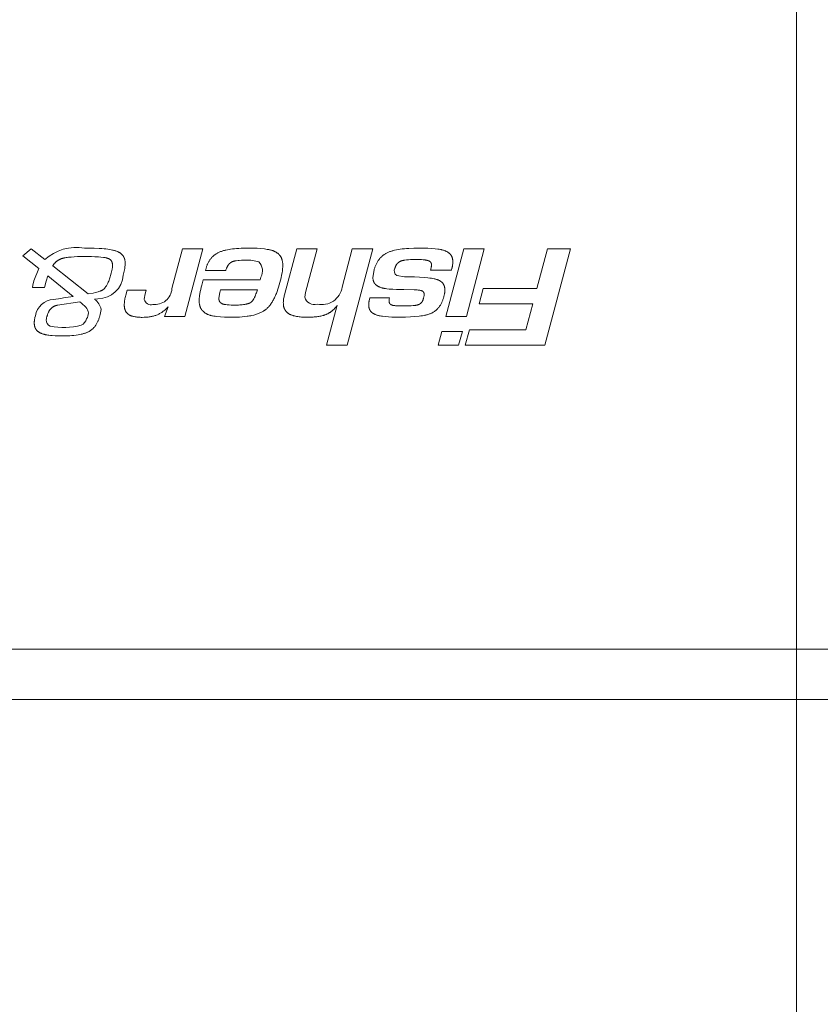
# Model space of a CAD drawing. Units: inches. Extents: x -1198 to -69, y -512 to 437.
# Tile 35 of 50: x -627.245 to -625.117, y 180.515 to 183.132. Entities that reach past the tile are written whole.
import ezdxf

# ---------------------------------------------------------------- set-up
doc = ezdxf.new("R2010")
doc.units = ezdxf.units.IN
doc.header["$MEASUREMENT"] = 0
for name, color, linetype, lineweight in [('0_Pen_No__7', 7, 'Continuous', 18), ('A-ANNO-DIMS', 2, 'Continuous', 18), ('A-EQPM', 60, 'Continuous', 18)]:
    doc.layers.add(name, color=color, linetype=linetype, lineweight=lineweight)
doc.styles.get("Standard").update_dxf_attribs({"font": 'arial.ttf'})
doc.dimstyles.get("Standard").update_dxf_attribs({"dimtxt": 6, "dimasz": 6, "dimexe": 0.18, "dimexo": 0.0625, "dimgap": 0.09, "dimtad": 0, "dimtih": 1, "dimtoh": 1, "dimdec": 0, "dimzin": 0, "dimdsep": 46, "dimlunit": 4, "dimtxsty": 'Standard', "dimblk": 'OBLIQUE', "dimcen": 0.09, "dimadec": 0, "dimazin": 0, "dimtfac": 1, "dimtdec": 0, "dimtofl": 0, "dimtmove": 0, "dimatfit": 3, "dimfxl": 1, "dimtolj": 1, "dimtzin": 0, "dimarcsym": 0})

# ---------------------------------------------------------------- blocks, each defined once
blk = doc.blocks.new('new block')
at = {"layer": '0_Pen_No__7'}
for p, q in [((-358.997, 99.109), (485.681, 99.109)), ((485.681, 95.73), (-358.997, 95.73)), ((-318.452, 68.7), (-316.721, 75.2)), ((-316.721, 75.2), (-311.349, 75.2)), ((-311.349, 75.2), (-311.629, 74.168)), ((-311.16, 74.266), (-310.904, 75.2)), ((-310.904, 75.2), (-309.527, 75.2)), ((-309.527, 75.2), (-309.782, 74.266)), ((-305.104, 68.7), (-303.373, 75.2)), ((-303.373, 75.2), (-301.997, 75.2)), ((-301.997, 75.2), (-302.715, 72.502)), ((-315.442, 74.168), (-315.906, 72.403)), ((-311.629, 74.168), (-315.442, 74.168)), ((-309.782, 74.266), (-311.16, 74.266)), ((-312.634, 68.7), (-311.429, 73.251)), ((-311.429, 73.251), (-310.05, 73.251)), ((-310.05, 73.251), (-311.257, 68.7)), ((-293.639, 68.7), (-292.433, 73.251)), ((-292.433, 73.251), (-291.056, 73.251)), ((-291.056, 73.251), (-291.311, 72.618)), ((-286.771, 72.786), (-286.716, 73.132)), ((-285.755, 72.627), (-285.462, 72.368)), ((-315.906, 72.403), (-312.288, 72.403)), ((-312.288, 72.403), (-312.567, 71.371)), ((-306.237, 72.004), (-306.225, 72.092)), ((-304.908, 72.004), (-306.237, 72.004)), ((-306.225, 72.092), (-306.213, 72.219)), ((-300.571, 71.634), (-300.522, 71.955)), ((-294.784, 71.634), (-294.723, 72.033)), ((-289.753, 71.731), (-289.691, 72.102)), ((-288.448, 71.819), (-288.533, 71.488)), ((-286.562, 72.059), (-286.329, 72.102)), ((-285.462, 72.368), (-285.335, 72.264)), ((-284.895, 71.907), (-283.174, 70.513)), ((-316.186, 71.371), (-316.892, 68.7)), ((-312.567, 71.371), (-316.186, 71.371)), ((-303.045, 71.283), (-303.727, 68.7)), ((-301.351, 68.7), (-300.571, 71.634)), ((-299.158, 71.789), (-299.974, 68.7)), ((-297.319, 71.458), (-294.833, 71.458)), ((-294.833, 71.458), (-294.784, 71.634)), ((-293.566, 71.146), (-293.663, 70.776)), ((-291.555, 71.379), (-292.26, 68.7)), ((-289.824, 71.488), (-289.753, 71.731)), ((-288.533, 71.488), (-289.824, 71.488)), ((-283.509, 69.837), (-285.894, 71.738)), ((-283.064, 70.877), (-282.962, 71.312)), ((-282.962, 71.312), (-282.141, 71.312)), ((-282.174, 71.152), (-282.242, 70.858)), ((-282.141, 71.312), (-282.174, 71.152)), ((-306.725, 70.503), (-307.261, 70.58)), ((-305.117, 70.62), (-305.202, 70.114)), ((-297.514, 70.776), (-297.561, 70.601)), ((-293.663, 70.776), (-297.514, 70.776)), ((-288.382, 70.016), (-288.272, 70.467)), ((-283.174, 70.513), (-283.064, 70.877)), ((-282.242, 70.858), (-282.564, 70.016)), ((-310.452, 70.006), (-310.417, 70.134)), ((-310.417, 70.134), (-309.003, 70.134)), ((-309.003, 70.134), (-309.04, 69.986)), ((-295.187, 70.152), (-293.822, 70.152)), ((-293.846, 70.065), (-293.858, 70.016)), ((-293.822, 70.152), (-293.846, 70.065)), ((-288.405, 69.686), (-288.382, 70.016)), ((-282.564, 70.016), (-281.486, 69.163)), ((-282.063, 68.7), (-282.973, 69.42)), ((-281.486, 69.163), (-282.063, 68.7)), ((-316.892, 68.7), (-318.452, 68.7)), ((-311.257, 68.7), (-312.634, 68.7)), ((-303.727, 68.7), (-305.104, 68.7)), ((-299.974, 68.7), (-301.351, 68.7)), ((-292.26, 68.7), (-293.639, 68.7))]:
    blk.add_line(p, q, dxfattribs=at)
blk.add_lwpolyline([(-333.701, 12.952), (460.296, 12.952), (460.296, 570.439), (-333.701, 570.439)], close=True, dxfattribs=at)
for points in [[(-286.716, 73.132), (-286.69, 73.224), (-286.662, 73.317), (-286.646, 73.362), (-286.63, 73.408), (-286.613, 73.453), (-286.595, 73.498), (-286.577, 73.543), (-286.557, 73.587), (-286.536, 73.63), (-286.514, 73.673), (-286.492, 73.716), (-286.468, 73.757), (-286.443, 73.799), (-286.417, 73.839), (-286.394, 73.873), (-286.37, 73.906), (-286.345, 73.938), (-286.32, 73.97), (-286.294, 74.001), (-286.266, 74.031), (-286.238, 74.06), (-286.209, 74.089), (-286.181, 74.115), (-286.152, 74.14), (-286.122, 74.164), (-286.091, 74.187), (-286.06, 74.209), (-286.028, 74.23), (-285.996, 74.25), (-285.963, 74.269), (-285.924, 74.29), (-285.885, 74.309), (-285.846, 74.327), (-285.806, 74.344), (-285.765, 74.36), (-285.724, 74.375), (-285.683, 74.389), (-285.641, 74.402), (-285.59, 74.417), (-285.538, 74.431), (-285.486, 74.444), (-285.434, 74.456), (-285.329, 74.478), (-285.223, 74.496), (-285.084, 74.517), (-284.943, 74.534), (-284.803, 74.547), (-284.662, 74.557), (-284.521, 74.564), (-284.379, 74.568), (-284.097, 74.572)], [(-284.097, 74.572), (-283.885, 74.569), (-283.673, 74.56), (-283.461, 74.545), (-283.355, 74.535), (-283.249, 74.523), (-283.177, 74.513), (-283.105, 74.502), (-283.033, 74.489), (-282.997, 74.481), (-282.962, 74.473), (-282.926, 74.464), (-282.891, 74.455), (-282.856, 74.444), (-282.821, 74.433), (-282.787, 74.42), (-282.753, 74.407), (-282.719, 74.393), (-282.686, 74.377), (-282.662, 74.365), (-282.639, 74.353), (-282.616, 74.34), (-282.594, 74.326), (-282.572, 74.312), (-282.55, 74.297), (-282.529, 74.282), (-282.508, 74.266), (-282.488, 74.249), (-282.478, 74.24), (-282.469, 74.232), (-282.459, 74.223), (-282.45, 74.214), (-282.441, 74.204), (-282.432, 74.195), (-282.423, 74.186), (-282.415, 74.176), (-282.407, 74.166), (-282.399, 74.156), (-282.391, 74.146), (-282.383, 74.135), (-282.376, 74.125), (-282.369, 74.114), (-282.362, 74.103), (-282.355, 74.091), (-282.349, 74.08), (-282.343, 74.068), (-282.337, 74.056), (-282.331, 74.044), (-282.326, 74.032), (-282.32, 74.02), (-282.315, 74.007), (-282.311, 73.995), (-282.306, 73.982), (-282.302, 73.969), (-282.298, 73.956), (-282.294, 73.943), (-282.291, 73.93), (-282.288, 73.917), (-282.282, 73.891), (-282.277, 73.864), (-282.273, 73.837), (-282.269, 73.81), (-282.267, 73.782), (-282.265, 73.755), (-282.264, 73.728), (-282.263, 73.701), (-282.263, 73.669), (-282.265, 73.638), (-282.267, 73.606), (-282.269, 73.575), (-282.273, 73.544), (-282.277, 73.513), (-282.282, 73.482), (-282.287, 73.451), (-282.299, 73.39), (-282.312, 73.329), (-282.342, 73.207)], [(-309.904, 71.926), (-309.878, 72.017), (-309.864, 72.062), (-309.849, 72.107), (-309.833, 72.152), (-309.816, 72.196), (-309.798, 72.24), (-309.78, 72.283), (-309.76, 72.326), (-309.739, 72.369), (-309.717, 72.411), (-309.694, 72.452), (-309.67, 72.493), (-309.645, 72.533), (-309.618, 72.572), (-309.591, 72.61), (-309.566, 72.643), (-309.54, 72.676), (-309.512, 72.707), (-309.484, 72.738), (-309.455, 72.768), (-309.426, 72.797), (-309.395, 72.825), (-309.363, 72.852), (-309.331, 72.878), (-309.298, 72.902), (-309.265, 72.926), (-309.23, 72.948), (-309.196, 72.969), (-309.16, 72.99), (-309.124, 73.009), (-309.087, 73.027), (-309.039, 73.05), (-308.989, 73.071), (-308.939, 73.091), (-308.888, 73.108), (-308.837, 73.125), (-308.785, 73.14), (-308.732, 73.154), (-308.68, 73.167), (-308.627, 73.179), (-308.573, 73.19), (-308.466, 73.209), (-308.359, 73.225), (-308.251, 73.239), (-307.955, 73.271), (-307.661, 73.292), (-307.323, 73.305), (-306.956, 73.31), (-306.678, 73.308), (-306.4, 73.299), (-306.169, 73.285), (-305.939, 73.266), (-305.777, 73.248), (-305.696, 73.237), (-305.615, 73.224), (-305.575, 73.216), (-305.535, 73.207), (-305.496, 73.198), (-305.456, 73.188), (-305.416, 73.176), (-305.377, 73.164), (-305.338, 73.15), (-305.299, 73.135), (-305.274, 73.124), (-305.249, 73.113), (-305.224, 73.102), (-305.199, 73.09), (-305.175, 73.077), (-305.151, 73.063), (-305.128, 73.049), (-305.105, 73.034), (-305.094, 73.026), (-305.083, 73.019), (-305.072, 73.01), (-305.062, 73.002), (-305.051, 72.994), (-305.041, 72.985), (-305.031, 72.976), (-305.021, 72.967), (-305.011, 72.958), (-305.002, 72.949), (-304.993, 72.939), (-304.984, 72.929), (-304.975, 72.919), (-304.967, 72.909), (-304.959, 72.899), (-304.951, 72.888), (-304.944, 72.877), (-304.937, 72.866), (-304.93, 72.855), (-304.923, 72.844), (-304.917, 72.832), (-304.911, 72.821), (-304.905, 72.809), (-304.899, 72.797), (-304.894, 72.785), (-304.889, 72.772), (-304.884, 72.76), (-304.88, 72.747), (-304.875, 72.735), (-304.871, 72.722), (-304.868, 72.709), (-304.864, 72.696), (-304.861, 72.683), (-304.858, 72.67), (-304.852, 72.643), (-304.847, 72.616), (-304.843, 72.589), (-304.84, 72.562), (-304.838, 72.535), (-304.837, 72.508), (-304.836, 72.481), (-304.836, 72.45), (-304.836, 72.42), (-304.838, 72.389), (-304.84, 72.359), (-304.843, 72.329), (-304.847, 72.299), (-304.852, 72.269), (-304.856, 72.239), (-304.867, 72.18), (-304.88, 72.121), (-304.908, 72.004)], [(-302.715, 72.502), (-302.674, 72.555), (-302.631, 72.607), (-302.588, 72.659), (-302.542, 72.709), (-302.495, 72.757), (-302.447, 72.804), (-302.422, 72.827), (-302.396, 72.85), (-302.371, 72.872), (-302.345, 72.893), (-302.321, 72.912), (-302.298, 72.93), (-302.274, 72.947), (-302.249, 72.965), (-302.225, 72.981), (-302.2, 72.998), (-302.175, 73.014), (-302.149, 73.029), (-302.124, 73.044), (-302.098, 73.059), (-302.072, 73.073), (-302.045, 73.086), (-302.018, 73.099), (-301.991, 73.112), (-301.964, 73.124), (-301.937, 73.135), (-301.905, 73.147), (-301.873, 73.159), (-301.841, 73.17), (-301.809, 73.181), (-301.776, 73.191), (-301.743, 73.2), (-301.677, 73.217), (-301.611, 73.231), (-301.544, 73.244), (-301.476, 73.256), (-301.409, 73.266), (-301.327, 73.277), (-301.244, 73.286), (-301.162, 73.293), (-301.079, 73.299), (-300.893, 73.307), (-300.706, 73.31), (-300.505, 73.307), (-300.404, 73.302), (-300.304, 73.296), (-300.218, 73.288), (-300.133, 73.279), (-300.048, 73.267), (-299.963, 73.254), (-299.897, 73.241), (-299.833, 73.227), (-299.8, 73.22), (-299.768, 73.211), (-299.736, 73.202), (-299.705, 73.193), (-299.673, 73.182), (-299.642, 73.171), (-299.611, 73.159), (-299.581, 73.146), (-299.551, 73.133), (-299.521, 73.118), (-299.492, 73.102), (-299.477, 73.094), (-299.463, 73.085), (-299.441, 73.071), (-299.419, 73.057), (-299.397, 73.041), (-299.376, 73.025), (-299.356, 73.009), (-299.335, 72.992), (-299.316, 72.974), (-299.297, 72.955), (-299.278, 72.936), (-299.261, 72.917), (-299.244, 72.897), (-299.236, 72.887), (-299.228, 72.876), (-299.22, 72.866), (-299.212, 72.855), (-299.205, 72.844), (-299.197, 72.833), (-299.19, 72.822), (-299.184, 72.811), (-299.177, 72.8), (-299.171, 72.788), (-299.164, 72.776), (-299.158, 72.763), (-299.152, 72.751), (-299.146, 72.738), (-299.14, 72.725), (-299.135, 72.712), (-299.13, 72.698), (-299.125, 72.685), (-299.121, 72.672), (-299.116, 72.658), (-299.109, 72.631), (-299.101, 72.603), (-299.095, 72.575), (-299.09, 72.547), (-299.085, 72.518), (-299.082, 72.49), (-299.079, 72.461), (-299.076, 72.433), (-299.075, 72.404), (-299.074, 72.375), (-299.073, 72.346), (-299.073, 72.311), (-299.074, 72.275), (-299.076, 72.239), (-299.079, 72.204), (-299.082, 72.169), (-299.086, 72.134), (-299.091, 72.099), (-299.096, 72.064), (-299.109, 71.994), (-299.123, 71.925), (-299.14, 71.857), (-299.158, 71.789)], [(-298.842, 70.97), (-298.801, 71.12), (-298.757, 71.27), (-298.71, 71.418), (-298.659, 71.565), (-298.603, 71.711), (-298.574, 71.783), (-298.543, 71.854), (-298.511, 71.925), (-298.477, 71.995), (-298.442, 72.064), (-298.406, 72.133), (-298.376, 72.186), (-298.345, 72.239), (-298.313, 72.292), (-298.28, 72.343), (-298.246, 72.394), (-298.211, 72.444), (-298.174, 72.493), (-298.135, 72.54), (-298.101, 72.581), (-298.066, 72.62), (-298.029, 72.659), (-297.992, 72.696), (-297.953, 72.733), (-297.913, 72.767), (-297.893, 72.784), (-297.872, 72.801), (-297.851, 72.817), (-297.83, 72.833), (-297.808, 72.849), (-297.785, 72.864), (-297.763, 72.879), (-297.739, 72.894), (-297.692, 72.922), (-297.645, 72.948), (-297.596, 72.974), (-297.546, 72.997), (-297.496, 73.02), (-297.446, 73.041), (-297.385, 73.064), (-297.324, 73.086), (-297.263, 73.107), (-297.201, 73.126), (-297.139, 73.144), (-297.076, 73.16), (-296.95, 73.19), (-296.869, 73.207), (-296.787, 73.222), (-296.705, 73.236), (-296.622, 73.249), (-296.457, 73.27), (-296.291, 73.286), (-296.125, 73.297), (-295.958, 73.305), (-295.625, 73.31)], [(-295.625, 73.31), (-295.36, 73.306), (-295.094, 73.296), (-294.828, 73.278), (-294.562, 73.251), (-294.474, 73.241), (-294.386, 73.229), (-294.299, 73.214), (-294.255, 73.205), (-294.212, 73.196), (-294.169, 73.186), (-294.127, 73.174), (-294.085, 73.161), (-294.043, 73.147), (-294.002, 73.132), (-293.982, 73.124), (-293.962, 73.115), (-293.942, 73.106), (-293.922, 73.097), (-293.902, 73.087), (-293.882, 73.077), (-293.855, 73.062), (-293.827, 73.045), (-293.8, 73.028), (-293.774, 73.01), (-293.748, 72.991), (-293.723, 72.972), (-293.699, 72.951), (-293.675, 72.93), (-293.652, 72.908), (-293.641, 72.897), (-293.63, 72.886), (-293.619, 72.874), (-293.608, 72.862), (-293.598, 72.85), (-293.588, 72.838), (-293.578, 72.826), (-293.568, 72.813), (-293.559, 72.801), (-293.55, 72.788), (-293.541, 72.775), (-293.533, 72.762), (-293.525, 72.748), (-293.517, 72.735), (-293.508, 72.719), (-293.5, 72.704), (-293.492, 72.688), (-293.484, 72.672), (-293.477, 72.655), (-293.47, 72.639), (-293.464, 72.622), (-293.458, 72.606), (-293.452, 72.589), (-293.447, 72.572), (-293.442, 72.555), (-293.437, 72.537), (-293.432, 72.52), (-293.428, 72.503), (-293.42, 72.467), (-293.414, 72.432), (-293.409, 72.396), (-293.404, 72.36), (-293.401, 72.324), (-293.398, 72.288), (-293.396, 72.251), (-293.395, 72.215), (-293.395, 72.179), (-293.396, 72.122), (-293.398, 72.065), (-293.402, 72.009), (-293.407, 71.953), (-293.413, 71.897), (-293.42, 71.842), (-293.437, 71.731), (-293.464, 71.584), (-293.495, 71.437), (-293.529, 71.291), (-293.566, 71.146)], [(-291.311, 72.618), (-291.264, 72.662), (-291.217, 72.706), (-291.168, 72.749), (-291.119, 72.792), (-291.069, 72.833), (-291.018, 72.873), (-290.966, 72.911), (-290.913, 72.949), (-290.866, 72.98), (-290.819, 73.011), (-290.771, 73.04), (-290.722, 73.068), (-290.673, 73.094), (-290.623, 73.119), (-290.572, 73.142), (-290.521, 73.164), (-290.468, 73.184), (-290.414, 73.203), (-290.359, 73.219), (-290.304, 73.235), (-290.249, 73.248), (-290.193, 73.26), (-290.137, 73.271), (-290.081, 73.281), (-290.017, 73.29), (-289.953, 73.298), (-289.889, 73.304), (-289.825, 73.31), (-289.755, 73.314), (-289.685, 73.317), (-289.545, 73.319), (-289.472, 73.319), (-289.4, 73.317), (-289.327, 73.313), (-289.255, 73.307), (-289.192, 73.301), (-289.13, 73.293), (-289.068, 73.283), (-289.006, 73.271), (-288.956, 73.26), (-288.907, 73.247), (-288.883, 73.24), (-288.859, 73.233), (-288.835, 73.225), (-288.811, 73.216), (-288.787, 73.207), (-288.764, 73.197), (-288.741, 73.187), (-288.718, 73.176), (-288.696, 73.164), (-288.674, 73.151), (-288.663, 73.145), (-288.653, 73.138), (-288.642, 73.131), (-288.632, 73.124), (-288.615, 73.111), (-288.598, 73.098), (-288.581, 73.085), (-288.565, 73.07), (-288.549, 73.056), (-288.534, 73.041), (-288.52, 73.025), (-288.505, 73.009), (-288.492, 72.992), (-288.478, 72.975), (-288.466, 72.958), (-288.454, 72.94), (-288.442, 72.922), (-288.432, 72.904), (-288.422, 72.885), (-288.412, 72.866), (-288.407, 72.855), (-288.402, 72.844), (-288.397, 72.832), (-288.393, 72.821), (-288.389, 72.81), (-288.385, 72.798), (-288.381, 72.786), (-288.377, 72.775), (-288.37, 72.751), (-288.364, 72.727), (-288.359, 72.703), (-288.355, 72.679), (-288.351, 72.654), (-288.347, 72.63), (-288.345, 72.605), (-288.343, 72.58), (-288.341, 72.556), (-288.34, 72.531), (-288.339, 72.481), (-288.34, 72.439), (-288.341, 72.396), (-288.344, 72.354), (-288.347, 72.312), (-288.352, 72.27), (-288.357, 72.229), (-288.363, 72.187), (-288.37, 72.145), (-288.386, 72.063), (-288.405, 71.981), (-288.426, 71.9), (-288.448, 71.819)], [(-285.335, 72.264), (-283.828, 72.5), (-283.806, 72.504), (-283.784, 72.508), (-283.762, 72.514), (-283.739, 72.519), (-283.717, 72.526), (-283.695, 72.533), (-283.673, 72.541), (-283.652, 72.549), (-283.631, 72.558), (-283.609, 72.567), (-283.59, 72.577), (-283.572, 72.587), (-283.553, 72.597), (-283.535, 72.608), (-283.517, 72.62), (-283.5, 72.632), (-283.483, 72.644), (-283.466, 72.657), (-283.45, 72.67), (-283.435, 72.684), (-283.42, 72.697), (-283.405, 72.712), (-283.391, 72.726), (-283.377, 72.741), (-283.364, 72.756), (-283.351, 72.772), (-283.338, 72.787), (-283.326, 72.804), (-283.313, 72.82), (-283.302, 72.837), (-283.29, 72.853), (-283.279, 72.871), (-283.268, 72.888), (-283.258, 72.905), (-283.248, 72.923), (-283.239, 72.94), (-283.22, 72.976), (-283.204, 73.012), (-283.188, 73.049), (-283.173, 73.086), (-283.159, 73.123), (-283.146, 73.161), (-283.134, 73.199), (-283.124, 73.235), (-283.115, 73.27), (-283.097, 73.342), (-283.082, 73.414), (-283.068, 73.487)], [(-307.236, 72.55), (-307.388, 72.549), (-307.54, 72.544), (-307.693, 72.536), (-307.846, 72.525), (-307.939, 72.516), (-307.986, 72.511), (-308.009, 72.507), (-308.032, 72.503), (-308.055, 72.499), (-308.078, 72.494), (-308.101, 72.489), (-308.123, 72.483), (-308.145, 72.476), (-308.167, 72.469), (-308.189, 72.461), (-308.2, 72.457), (-308.211, 72.452), (-308.224, 72.446), (-308.238, 72.44), (-308.251, 72.433), (-308.264, 72.426), (-308.277, 72.418), (-308.29, 72.411), (-308.302, 72.403), (-308.315, 72.394), (-308.327, 72.386), (-308.338, 72.377), (-308.35, 72.367), (-308.361, 72.358), (-308.372, 72.348), (-308.383, 72.337), (-308.393, 72.326), (-308.403, 72.315), (-308.413, 72.304), (-308.422, 72.292), (-308.431, 72.28), (-308.439, 72.267), (-308.447, 72.255), (-308.455, 72.242), (-308.463, 72.228), (-308.47, 72.215), (-308.477, 72.201), (-308.483, 72.188), (-308.489, 72.174), (-308.495, 72.159), (-308.5, 72.145), (-308.505, 72.131), (-308.51, 72.117), (-308.515, 72.102), (-308.522, 72.075), (-308.529, 72.048), (-308.535, 72.02), (-308.568, 71.844), (-308.572, 71.825), (-308.575, 71.807), (-308.577, 71.788), (-308.578, 71.769), (-308.578, 71.75), (-308.577, 71.736), (-308.576, 71.721), (-308.574, 71.711), (-308.572, 71.701), (-308.57, 71.691), (-308.567, 71.681), (-308.564, 71.671), (-308.561, 71.662), (-308.557, 71.652), (-308.552, 71.643), (-308.548, 71.634), (-308.543, 71.625), (-308.538, 71.616), (-308.532, 71.608), (-308.526, 71.6), (-308.516, 71.589), (-308.508, 71.58), (-308.499, 71.572), (-308.489, 71.563), (-308.478, 71.556), (-308.467, 71.549), (-308.455, 71.542), (-308.444, 71.536), (-308.431, 71.531), (-308.413, 71.523), (-308.4, 71.519), (-308.387, 71.514), (-308.374, 71.511), (-308.36, 71.507), (-308.347, 71.504), (-308.32, 71.498), (-308.294, 71.493), (-308.268, 71.488), (-308.243, 71.484), (-308.217, 71.48), (-308.166, 71.474), (-308.115, 71.47), (-308.064, 71.466), (-307.913, 71.461), (-307.2, 71.448)], [(-306.213, 72.219), (-306.213, 72.23), (-306.213, 72.242), (-306.214, 72.253), (-306.215, 72.265), (-306.217, 72.277), (-306.219, 72.288), (-306.221, 72.3), (-306.224, 72.311), (-306.227, 72.322), (-306.23, 72.333), (-306.234, 72.344), (-306.239, 72.354), (-306.244, 72.365), (-306.249, 72.375), (-306.255, 72.384), (-306.261, 72.394), (-306.268, 72.402), (-306.275, 72.411), (-306.283, 72.419), (-306.291, 72.426), (-306.299, 72.433), (-306.308, 72.44), (-306.317, 72.447), (-306.326, 72.453), (-306.336, 72.459), (-306.346, 72.465), (-306.356, 72.47), (-306.366, 72.475), (-306.376, 72.48), (-306.387, 72.484), (-306.397, 72.488), (-306.408, 72.492), (-306.427, 72.498), (-306.445, 72.504), (-306.464, 72.509), (-306.483, 72.513), (-306.502, 72.517), (-306.521, 72.52), (-306.54, 72.523), (-306.559, 72.526), (-306.597, 72.529), (-306.635, 72.532), (-306.974, 72.546), (-307.236, 72.55)], [(-295.807, 72.492), (-295.973, 72.49), (-296.056, 72.488), (-296.139, 72.484), (-296.222, 72.478), (-296.304, 72.47), (-296.386, 72.46), (-296.468, 72.448), (-296.526, 72.437), (-296.585, 72.424), (-296.614, 72.417), (-296.643, 72.41), (-296.671, 72.401), (-296.7, 72.392), (-296.722, 72.385), (-296.744, 72.377), (-296.765, 72.369), (-296.787, 72.36), (-296.797, 72.355), (-296.808, 72.35), (-296.818, 72.345), (-296.828, 72.339), (-296.838, 72.334), (-296.848, 72.328), (-296.858, 72.322), (-296.867, 72.315), (-296.876, 72.309), (-296.885, 72.303), (-296.893, 72.296), (-296.902, 72.29), (-296.91, 72.283), (-296.918, 72.275), (-296.926, 72.268), (-296.934, 72.261), (-296.941, 72.253), (-296.949, 72.245), (-296.964, 72.229), (-296.978, 72.213), (-296.992, 72.196), (-297.008, 72.175), (-297.024, 72.153), (-297.04, 72.13), (-297.054, 72.107), (-297.069, 72.084), (-297.082, 72.061), (-297.109, 72.013), (-297.126, 71.98), (-297.142, 71.947), (-297.158, 71.913), (-297.173, 71.879), (-297.201, 71.811), (-297.228, 71.741), (-297.253, 71.671), (-297.276, 71.6), (-297.319, 71.458)], [(-294.723, 72.033), (-294.723, 72.048), (-294.724, 72.063), (-294.725, 72.079), (-294.726, 72.094), (-294.728, 72.11), (-294.73, 72.125), (-294.732, 72.14), (-294.736, 72.155), (-294.739, 72.17), (-294.743, 72.185), (-294.748, 72.2), (-294.753, 72.214), (-294.759, 72.228), (-294.766, 72.242), (-294.773, 72.255), (-294.781, 72.268), (-294.789, 72.279), (-294.797, 72.29), (-294.806, 72.3), (-294.815, 72.31), (-294.825, 72.32), (-294.835, 72.329), (-294.846, 72.338), (-294.857, 72.347), (-294.868, 72.355), (-294.88, 72.363), (-294.891, 72.37), (-294.904, 72.377), (-294.916, 72.384), (-294.928, 72.391), (-294.941, 72.397), (-294.954, 72.403), (-294.963, 72.407), (-294.973, 72.411), (-294.992, 72.418), (-295.012, 72.425), (-295.032, 72.431), (-295.052, 72.436), (-295.072, 72.441), (-295.092, 72.445), (-295.113, 72.449), (-295.133, 72.453), (-295.154, 72.456), (-295.195, 72.461), (-295.277, 72.469), (-295.41, 72.479), (-295.542, 72.486), (-295.675, 72.491), (-295.807, 72.492)], [(-307.261, 70.58), (-307.93, 70.588), (-308.264, 70.602), (-308.598, 70.625), (-308.835, 70.648), (-308.954, 70.663), (-309.072, 70.68), (-309.159, 70.695), (-309.246, 70.712), (-309.29, 70.722), (-309.333, 70.732), (-309.375, 70.744), (-309.418, 70.757), (-309.45, 70.767), (-309.481, 70.779), (-309.513, 70.791), (-309.543, 70.804), (-309.574, 70.818), (-309.604, 70.833), (-309.619, 70.841), (-309.634, 70.849), (-309.648, 70.857), (-309.663, 70.866), (-309.675, 70.874), (-309.687, 70.882), (-309.699, 70.89), (-309.711, 70.898), (-309.723, 70.907), (-309.734, 70.916), (-309.746, 70.925), (-309.757, 70.934), (-309.768, 70.944), (-309.778, 70.954), (-309.789, 70.964), (-309.799, 70.974), (-309.809, 70.984), (-309.819, 70.995), (-309.828, 71.006), (-309.837, 71.017), (-309.846, 71.029), (-309.854, 71.04), (-309.862, 71.052), (-309.87, 71.064), (-309.877, 71.076), (-309.884, 71.088), (-309.891, 71.101), (-309.898, 71.113), (-309.904, 71.126), (-309.91, 71.139), (-309.916, 71.152), (-309.921, 71.165), (-309.926, 71.179), (-309.931, 71.192), (-309.936, 71.206), (-309.94, 71.22), (-309.944, 71.234), (-309.948, 71.248), (-309.952, 71.262), (-309.955, 71.276), (-309.961, 71.304), (-309.966, 71.333), (-309.97, 71.362), (-309.973, 71.39), (-309.976, 71.419), (-309.977, 71.448), (-309.977, 71.479), (-309.977, 71.509), (-309.976, 71.54), (-309.973, 71.57), (-309.97, 71.6), (-309.967, 71.63), (-309.963, 71.66), (-309.958, 71.69), (-309.946, 71.75), (-309.933, 71.809), (-309.904, 71.926)], [(-307.2, 71.448), (-306.952, 71.446), (-306.705, 71.438), (-306.457, 71.425), (-306.209, 71.405), (-306.049, 71.387), (-305.969, 71.376), (-305.89, 71.363), (-305.851, 71.355), (-305.811, 71.347), (-305.772, 71.337), (-305.733, 71.327), (-305.694, 71.315), (-305.656, 71.303), (-305.617, 71.289), (-305.579, 71.274), (-305.554, 71.263), (-305.529, 71.252), (-305.504, 71.24), (-305.48, 71.228), (-305.455, 71.215), (-305.432, 71.201), (-305.409, 71.187), (-305.386, 71.171), (-305.375, 71.164), (-305.364, 71.156), (-305.353, 71.147), (-305.342, 71.139), (-305.332, 71.13), (-305.322, 71.122), (-305.312, 71.113), (-305.302, 71.103), (-305.292, 71.094), (-305.283, 71.084), (-305.274, 71.075), (-305.265, 71.065), (-305.256, 71.055), (-305.248, 71.044), (-305.24, 71.034), (-305.232, 71.023), (-305.225, 71.012), (-305.217, 71.001), (-305.211, 70.99), (-305.204, 70.978), (-305.198, 70.967), (-305.191, 70.955), (-305.186, 70.943), (-305.18, 70.931), (-305.175, 70.919), (-305.17, 70.907), (-305.165, 70.895), (-305.16, 70.882), (-305.156, 70.87), (-305.152, 70.857), (-305.148, 70.844), (-305.144, 70.831), (-305.141, 70.818), (-305.138, 70.805), (-305.135, 70.792), (-305.132, 70.779), (-305.127, 70.752), (-305.123, 70.726), (-305.12, 70.699), (-305.118, 70.673), (-305.117, 70.647), (-305.117, 70.62)], [(-285.894, 71.738), (-286.234, 71.675), (-286.403, 71.638), (-286.486, 71.617), (-286.57, 71.594), (-286.625, 71.577), (-286.679, 71.559), (-286.706, 71.549), (-286.733, 71.539), (-286.76, 71.528), (-286.786, 71.517), (-286.806, 71.507), (-286.826, 71.497), (-286.846, 71.487), (-286.865, 71.476), (-286.884, 71.465), (-286.893, 71.459), (-286.902, 71.453), (-286.911, 71.447), (-286.92, 71.44), (-286.929, 71.434), (-286.937, 71.427), (-286.946, 71.42), (-286.955, 71.412), (-286.963, 71.405), (-286.971, 71.397), (-286.979, 71.389), (-286.987, 71.381), (-287.003, 71.364), (-287.018, 71.347), (-287.032, 71.329), (-287.046, 71.311), (-287.06, 71.293), (-287.078, 71.268), (-287.095, 71.243), (-287.112, 71.218), (-287.128, 71.193), (-287.159, 71.142), (-287.188, 71.09), (-287.207, 71.055), (-287.225, 71.02), (-287.258, 70.949), (-287.29, 70.876), (-287.32, 70.803), (-287.347, 70.729), (-287.372, 70.654), (-287.396, 70.579), (-287.417, 70.503)], [(-293.858, 70.016), (-293.869, 69.973), (-293.882, 69.929), (-293.895, 69.886), (-293.91, 69.844), (-293.925, 69.801), (-293.942, 69.759), (-293.96, 69.717), (-293.978, 69.676), (-293.998, 69.635), (-294.018, 69.595), (-294.04, 69.555), (-294.063, 69.516), (-294.087, 69.478), (-294.112, 69.441), (-294.139, 69.404), (-294.166, 69.368), (-294.193, 69.335), (-294.221, 69.303), (-294.25, 69.271), (-294.28, 69.241), (-294.311, 69.211), (-294.343, 69.182), (-294.375, 69.154), (-294.409, 69.127), (-294.443, 69.101), (-294.478, 69.076), (-294.513, 69.052), (-294.549, 69.028), (-294.586, 69.006), (-294.623, 68.985), (-294.66, 68.964), (-294.698, 68.945), (-294.746, 68.922), (-294.795, 68.9), (-294.844, 68.88), (-294.894, 68.862), (-294.944, 68.844), (-294.994, 68.828), (-295.045, 68.813), (-295.097, 68.799), (-295.148, 68.786), (-295.2, 68.774), (-295.305, 68.753), (-295.41, 68.734), (-295.515, 68.718), (-295.651, 68.699), (-295.788, 68.684), (-295.924, 68.671), (-296.06, 68.661), (-296.22, 68.653), (-296.379, 68.647), (-296.698, 68.642), (-297, 68.645), (-297.151, 68.65), (-297.301, 68.658), (-297.553, 68.677), (-297.806, 68.703), (-297.899, 68.714), (-297.992, 68.728), (-298.084, 68.743), (-298.13, 68.752), (-298.175, 68.762), (-298.221, 68.773), (-298.265, 68.785), (-298.31, 68.798), (-298.354, 68.813), (-298.398, 68.829), (-298.419, 68.837), (-298.441, 68.846), (-298.462, 68.856), (-298.483, 68.866), (-298.504, 68.876), (-298.525, 68.887), (-298.554, 68.902), (-298.583, 68.919), (-298.611, 68.937), (-298.639, 68.955), (-298.666, 68.975), (-298.692, 68.995), (-298.718, 69.016), (-298.743, 69.038), (-298.755, 69.049), (-298.767, 69.061), (-298.779, 69.072), (-298.791, 69.084), (-298.802, 69.096), (-298.813, 69.109), (-298.824, 69.121), (-298.834, 69.134), (-298.845, 69.147), (-298.855, 69.16), (-298.864, 69.173), (-298.874, 69.186), (-298.883, 69.2), (-298.892, 69.214), (-298.901, 69.228), (-298.909, 69.242), (-298.917, 69.257), (-298.925, 69.272), (-298.933, 69.288), (-298.94, 69.304), (-298.947, 69.32), (-298.954, 69.336), (-298.96, 69.352), (-298.966, 69.369), (-298.972, 69.385), (-298.978, 69.402), (-298.988, 69.435), (-298.997, 69.469), (-299.004, 69.503), (-299.012, 69.542), (-299.019, 69.582), (-299.024, 69.621), (-299.029, 69.661), (-299.032, 69.701), (-299.035, 69.741), (-299.036, 69.781), (-299.036, 69.82), (-299.035, 69.882), (-299.033, 69.943), (-299.028, 70.004), (-299.022, 70.065), (-299.015, 70.126), (-299.007, 70.187), (-298.988, 70.309), (-298.957, 70.475), (-298.922, 70.641), (-298.842, 70.97)], [(-287.417, 70.503), (-287.464, 70.331), (-287.506, 70.158), (-287.524, 70.07), (-287.532, 70.026), (-287.539, 69.982), (-287.544, 69.938), (-287.546, 69.915), (-287.548, 69.893), (-287.549, 69.871), (-287.55, 69.848), (-287.55, 69.825), (-287.549, 69.802), (-287.549, 69.782), (-287.547, 69.761), (-287.545, 69.74), (-287.542, 69.719), (-287.539, 69.698), (-287.535, 69.677), (-287.531, 69.657), (-287.528, 69.647), (-287.526, 69.636), (-287.523, 69.626), (-287.52, 69.616), (-287.516, 69.607), (-287.513, 69.597), (-287.509, 69.587), (-287.505, 69.578), (-287.501, 69.568), (-287.497, 69.559), (-287.493, 69.55), (-287.488, 69.54), (-287.483, 69.532), (-287.478, 69.523), (-287.473, 69.514), (-287.467, 69.505), (-287.461, 69.497), (-287.455, 69.489), (-287.443, 69.474), (-287.43, 69.459), (-287.416, 69.445), (-287.401, 69.431), (-287.386, 69.418), (-287.37, 69.406), (-287.354, 69.395), (-287.337, 69.384), (-287.327, 69.378), (-287.317, 69.373), (-287.308, 69.367), (-287.298, 69.362), (-287.287, 69.357), (-287.277, 69.352), (-287.267, 69.348), (-287.257, 69.343), (-287.236, 69.335), (-287.214, 69.328), (-287.193, 69.321), (-287.171, 69.314), (-287.142, 69.306), (-287.113, 69.3), (-287.083, 69.293), (-287.054, 69.288), (-286.994, 69.279), (-286.934, 69.271), (-286.767, 69.253), (-286.6, 69.24), (-286.36, 69.226), (-286.12, 69.219), (-285.639, 69.214)], [(-305.202, 70.114), (-305.215, 70.067), (-305.229, 70.021), (-305.243, 69.974), (-305.259, 69.928), (-305.276, 69.882), (-305.294, 69.837), (-305.312, 69.791), (-305.332, 69.747), (-305.353, 69.703), (-305.375, 69.659), (-305.398, 69.616), (-305.422, 69.574), (-305.448, 69.532), (-305.474, 69.491), (-305.502, 69.451), (-305.531, 69.412), (-305.558, 69.377), (-305.587, 69.343), (-305.616, 69.309), (-305.647, 69.277), (-305.678, 69.245), (-305.71, 69.214), (-305.743, 69.185), (-305.777, 69.156), (-305.812, 69.128), (-305.848, 69.101), (-305.885, 69.076), (-305.922, 69.051), (-305.961, 69.028), (-305.999, 69.005), (-306.039, 68.984), (-306.079, 68.963), (-306.125, 68.942), (-306.171, 68.921), (-306.219, 68.902), (-306.266, 68.884), (-306.314, 68.867), (-306.363, 68.851), (-306.412, 68.836), (-306.461, 68.823), (-306.521, 68.806), (-306.582, 68.792), (-306.704, 68.765), (-306.827, 68.742), (-306.95, 68.722), (-307.098, 68.702), (-307.247, 68.686), (-307.396, 68.673), (-307.545, 68.662), (-307.883, 68.647), (-308.248, 68.642), (-308.538, 68.645), (-308.829, 68.654), (-309.073, 68.67), (-309.317, 68.691), (-309.494, 68.71), (-309.583, 68.722), (-309.671, 68.737), (-309.715, 68.746), (-309.758, 68.755), (-309.802, 68.766), (-309.845, 68.778), (-309.888, 68.79), (-309.93, 68.805), (-309.973, 68.82), (-310.014, 68.837), (-310.042, 68.849), (-310.069, 68.862), (-310.096, 68.875), (-310.122, 68.889), (-310.149, 68.904), (-310.174, 68.919), (-310.199, 68.936), (-310.224, 68.953), (-310.236, 68.961), (-310.248, 68.97), (-310.259, 68.979), (-310.271, 68.989), (-310.282, 68.998), (-310.293, 69.008), (-310.304, 69.018), (-310.314, 69.028), (-310.325, 69.039), (-310.335, 69.049), (-310.344, 69.06), (-310.354, 69.071), (-310.363, 69.082), (-310.372, 69.094), (-310.381, 69.105), (-310.389, 69.117), (-310.397, 69.129), (-310.405, 69.141), (-310.412, 69.153), (-310.419, 69.165), (-310.426, 69.177), (-310.432, 69.19), (-310.438, 69.202), (-310.444, 69.215), (-310.45, 69.228), (-310.455, 69.241), (-310.46, 69.254), (-310.465, 69.268), (-310.47, 69.281), (-310.474, 69.295), (-310.478, 69.308), (-310.482, 69.322), (-310.49, 69.35), (-310.496, 69.378), (-310.501, 69.406), (-310.505, 69.434), (-310.509, 69.463), (-310.512, 69.491), (-310.514, 69.52), (-310.515, 69.548), (-310.515, 69.575), (-310.515, 69.602), (-310.514, 69.629), (-310.512, 69.656), (-310.508, 69.709), (-310.502, 69.762), (-310.493, 69.824), (-310.488, 69.855), (-310.483, 69.886), (-310.476, 69.916), (-310.469, 69.947), (-310.461, 69.977), (-310.452, 70.006)], [(-309.04, 69.986), (-309.048, 69.96), (-309.055, 69.934), (-309.062, 69.907), (-309.064, 69.894), (-309.067, 69.881), (-309.069, 69.867), (-309.072, 69.854), (-309.073, 69.84), (-309.075, 69.827), (-309.075, 69.813), (-309.076, 69.799), (-309.076, 69.786), (-309.076, 69.772), (-309.075, 69.76), (-309.074, 69.749), (-309.072, 69.737), (-309.07, 69.726), (-309.068, 69.714), (-309.066, 69.703), (-309.063, 69.692), (-309.059, 69.68), (-309.056, 69.67), (-309.051, 69.659), (-309.047, 69.648), (-309.042, 69.638), (-309.036, 69.628), (-309.031, 69.618), (-309.024, 69.609), (-309.018, 69.6), (-309.01, 69.59), (-309.001, 69.581), (-308.992, 69.572), (-308.982, 69.563), (-308.973, 69.555), (-308.962, 69.547), (-308.951, 69.54), (-308.94, 69.533), (-308.929, 69.526), (-308.917, 69.52), (-308.906, 69.514), (-308.894, 69.509), (-308.881, 69.503), (-308.869, 69.498), (-308.857, 69.494), (-308.844, 69.489), (-308.824, 69.482), (-308.803, 69.476), (-308.783, 69.471), (-308.762, 69.465), (-308.742, 69.461), (-308.721, 69.457), (-308.7, 69.453), (-308.679, 69.449), (-308.638, 69.444), (-308.596, 69.439), (-308.512, 69.432), (-308.396, 69.423), (-308.28, 69.417), (-308.142, 69.413), (-308.003, 69.412), (-307.832, 69.414), (-307.661, 69.42), (-307.519, 69.429), (-307.377, 69.441), (-307.275, 69.453), (-307.224, 69.461), (-307.199, 69.465), (-307.174, 69.47), (-307.149, 69.475), (-307.125, 69.481), (-307.1, 69.487), (-307.076, 69.494), (-307.052, 69.502), (-307.028, 69.51), (-307.004, 69.519), (-306.992, 69.524), (-306.981, 69.529), (-306.964, 69.537), (-306.948, 69.545), (-306.931, 69.554), (-306.915, 69.563), (-306.899, 69.573), (-306.884, 69.583), (-306.868, 69.594), (-306.853, 69.604), (-306.839, 69.616), (-306.824, 69.628), (-306.81, 69.64), (-306.797, 69.652), (-306.783, 69.665), (-306.771, 69.679), (-306.758, 69.692), (-306.746, 69.706), (-306.74, 69.715), (-306.733, 69.723), (-306.727, 69.731), (-306.721, 69.74), (-306.709, 69.757), (-306.698, 69.775), (-306.688, 69.793), (-306.678, 69.811), (-306.668, 69.83), (-306.659, 69.849), (-306.65, 69.868), (-306.642, 69.887), (-306.635, 69.907), (-306.628, 69.927), (-306.621, 69.946), (-306.614, 69.966), (-306.603, 70.006)], [(-296.562, 69.46), (-296.408, 69.462), (-296.254, 69.467), (-296.099, 69.477), (-296.022, 69.484), (-295.896, 69.498), (-295.848, 69.504), (-295.801, 69.513), (-295.777, 69.517), (-295.754, 69.523), (-295.731, 69.528), (-295.708, 69.535), (-295.685, 69.542), (-295.662, 69.549), (-295.64, 69.557), (-295.629, 69.562), (-295.618, 69.567), (-295.608, 69.571), (-295.597, 69.577), (-295.586, 69.582), (-295.576, 69.587), (-295.559, 69.597), (-295.543, 69.607), (-295.527, 69.617), (-295.512, 69.628), (-295.496, 69.639), (-295.481, 69.651), (-295.467, 69.664), (-295.452, 69.677), (-295.438, 69.69), (-295.425, 69.703), (-295.411, 69.717), (-295.398, 69.732), (-295.386, 69.746), (-295.374, 69.761), (-295.362, 69.777), (-295.351, 69.792), (-295.336, 69.813), (-295.323, 69.834), (-295.31, 69.855), (-295.298, 69.876), (-295.286, 69.898), (-295.275, 69.921), (-295.264, 69.943), (-295.254, 69.966), (-295.244, 69.989), (-295.235, 70.012), (-295.218, 70.058), (-295.202, 70.105), (-295.187, 70.152)], [(-285.639, 69.214), (-285.191, 69.22), (-284.967, 69.23), (-284.743, 69.246), (-284.578, 69.262), (-284.495, 69.273), (-284.413, 69.285), (-284.35, 69.296), (-284.287, 69.308), (-284.255, 69.315), (-284.224, 69.323), (-284.193, 69.331), (-284.162, 69.34), (-284.137, 69.348), (-284.111, 69.356), (-284.086, 69.365), (-284.061, 69.375), (-284.036, 69.385), (-284.012, 69.395), (-283.987, 69.406), (-283.963, 69.418), (-283.94, 69.43), (-283.918, 69.442), (-283.895, 69.455), (-283.873, 69.468), (-283.851, 69.482), (-283.83, 69.497), (-283.809, 69.511), (-283.788, 69.527), (-283.767, 69.543), (-283.747, 69.56), (-283.727, 69.577), (-283.708, 69.594), (-283.689, 69.613), (-283.67, 69.631), (-283.652, 69.65), (-283.634, 69.67), (-283.617, 69.689), (-283.6, 69.71), (-283.583, 69.73), (-283.567, 69.751), (-283.552, 69.772), (-283.537, 69.794), (-283.523, 69.815), (-283.509, 69.837)], [(-285.652, 68.637), (-285.985, 68.64), (-286.317, 68.648), (-286.65, 68.664), (-286.815, 68.676), (-286.981, 68.691), (-287.101, 68.704), (-287.221, 68.72), (-287.341, 68.737), (-287.461, 68.758), (-287.551, 68.777), (-287.596, 68.787), (-287.641, 68.798), (-287.685, 68.809), (-287.729, 68.822), (-287.773, 68.836), (-287.817, 68.852), (-287.851, 68.865), (-287.884, 68.878), (-287.917, 68.893), (-287.95, 68.909), (-287.982, 68.926), (-287.998, 68.935), (-288.013, 68.944), (-288.029, 68.953), (-288.044, 68.963), (-288.059, 68.973), (-288.074, 68.983), (-288.087, 68.993), (-288.1, 69.003), (-288.113, 69.013), (-288.126, 69.023), (-288.138, 69.034), (-288.15, 69.044), (-288.162, 69.056), (-288.174, 69.067), (-288.185, 69.079), (-288.197, 69.09), (-288.208, 69.102), (-288.218, 69.115), (-288.229, 69.127), (-288.239, 69.14), (-288.249, 69.153), (-288.258, 69.166), (-288.267, 69.18), (-288.277, 69.195), (-288.285, 69.209), (-288.294, 69.224), (-288.302, 69.239), (-288.31, 69.254), (-288.317, 69.269), (-288.324, 69.285), (-288.331, 69.301), (-288.338, 69.316), (-288.344, 69.332), (-288.35, 69.348), (-288.355, 69.365), (-288.361, 69.381), (-288.365, 69.398), (-288.37, 69.414), (-288.374, 69.431), (-288.378, 69.448), (-288.386, 69.481), (-288.392, 69.515), (-288.396, 69.549), (-288.4, 69.584), (-288.403, 69.618), (-288.404, 69.652), (-288.405, 69.686)]]:
    blk.add_lwpolyline(points, dxfattribs=at)
for centre, radius, start, end in [((-285.125, 73.216), 0.705, 115.53732, 162.79084), ((-284.239, 68.997), 4.998, 79.64276, 103.77478), ((-283.503, 73.51), 0.436, 356.91901, 68.05296), ((-285.264, 73.054), 0.65, 145.25463, 220.99631), ((-283.634, 73.41), 1.308, 273.24586, 351.11338), ((-301.668, 71.062), 1.395, 77.4021, 170.88599), ((-290.392, 71.293), 1.166, 83.68162, 175.75797), ((-290.137, 72.017), 0.454, 10.86555, 106.28223), ((-285.754, 72.959), 1.031, 189.64199, 236.13883), ((-301.171, 71.779), 0.672, 15.22031, 106.60136), ((-286.56, 70.341), 1.717, 90.06134, 175.7929), ((-278.463, 32.809), 39.624, 97.39024, 99.34153), ((-306.942, 70.187), 0.384, 332.01224, 55.5965), ((-296.818, 70.185), 0.852, 150.76729, 225.46616), ((-296.683, 71.747), 2.29, 251.35459, 273.04349), ((-285.137, 71.848), 3.252, 260.88312, 311.69618)]:
    blk.add_arc(centre, radius, start, end, dxfattribs=at)
blk = doc.blocks.new('_Oblique')
at = {"color": 0, "linetype": 'ByBlock', "lineweight": -2}
blk.add_line((-0.5, -0.5), (0.5, 0.5), dxfattribs=at)
blk = doc.blocks.new('*D56')
at = {"layer": 'A-ANNO-DIMS', "color": 0, "lineweight": -2, "ltscale": 10, "transparency": 16777216}
for p, q in [((-618.3394, 257.2277), (-603.8219, 257.2277)), ((-604.0019, 257.2277), (-604.0019, 212.422)), ((-604.0019, 161.2277), (-604.0019, 206.0333)), ((-618.3394, 161.2277), (-603.8219, 161.2277))]:
    blk.add_line(p, q, dxfattribs=at)
at = {"layer": 'DEFPOINTS', "color": 0, "ltscale": 10, "transparency": 16777216}
for p in [(-618.4019, 257.2277), (-604.0019, 257.2277), (-618.4019, 161.2277)]:
    blk.add_point(p, dxfattribs=at)
at = {"layer": 'A-ANNO-DIMS', "color": 0, "lineweight": -2, "ltscale": 10, "transparency": 16777216, "xscale": 6, "yscale": 6, "zscale": 6}
for p, rotation in [((-604.0019, 257.2277), 90), ((-604.0019, 161.2277), 270)]:
    blk.add_blockref('_Oblique', p, dxfattribs=dict(at, rotation=rotation))
at = {"layer": 'A-ANNO-DIMS', "color": 0, "ltscale": 10, "transparency": 16777216, "insert": (-604.0019, 209.2277), "char_height": 6, "attachment_point": 5}
blk.add_mtext('\\A1;COUNTER 96 TYP.', dxfattribs=at)

msp = doc.modelspace()

# ---------------------------------------------------------------- block references
at = {"layer": 'A-EQPM', "xscale": 0.0393700787401575, "yscale": 0.0393700787401575, "zscale": 0.0393700787401575, "rotation": 180}
msp.add_blockref('new block', (-638.3186, 185.2277), dxfattribs=at)

# ---------------------------------------------------------------- dimensions: what is measured, and where the dimension line sits
at = {"layer": 'A-ANNO-DIMS', "ltscale": 10}
dim = msp.add_linear_dim(base=(-604.0019, 257.2277), p1=(-618.4019, 161.2277), p2=(-618.4019, 257.2277), angle=90, text='COUNTER <> TYP.', dimstyle='Standard', override={"dimdec": 0, "dimlfac": 1, "dimrnd": 0, "dimzin": 0, "dimdsep": 46, "dimlunit": 2}, dxfattribs=at)
dim.commit()
dim.dimension.update_dxf_attribs({"geometry": '*D56', "text_midpoint": (-604.0019, 209.2277)})

doc.saveas('drawing.dxf')
